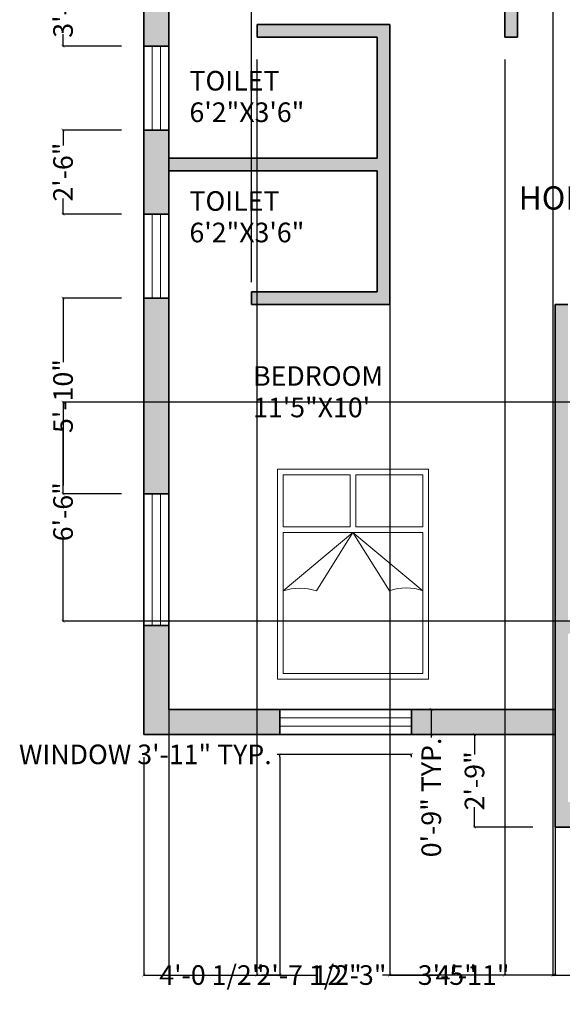
# Model space of a CAD drawing. Units: inches. Extents: x 98 to 545, y 56 to 703.
# Tile 1 of 4: x 98 to 292, y 56 to 408. Entities that reach past the tile are written whole.
import ezdxf

# ---------------------------------------------------------------- set-up
doc = ezdxf.new("R2010")
doc.units = ezdxf.units.IN
doc.header["$MEASUREMENT"] = 0
for name, color, linetype, lineweight in [('A-ANNO-DIMS', 2, 'Continuous', 18), ('A-ANNO-TEXT', 7, 'Continuous', 25), ('A-AREA-IDEN', 7, 'Continuous', 25), ('A-GLAZ', 4, 'Continuous', 18), ('A-WALL', 7, 'Continuous', 35), ('Furniture', 7, 'Continuous', 15)]:
    doc.layers.add(name, color=color, linetype=linetype, lineweight=lineweight)
doc.layers.add('A-WALL-PATT', color=18, linetype='Continuous', lineweight=13, true_color=0x000000)
doc.styles.get("Standard").update_dxf_attribs({"font": 'arial.ttf'})
doc.dimstyles.get("Standard").update_dxf_attribs({"dimtxt": 7, "dimasz": 1, "dimexe": 0.183, "dimexo": 8, "dimgap": 0.09, "dimtad": 0, "dimdec": 4, "dimzin": 0, "dimdsep": 46, "dimlunit": 3, "dimtxsty": 'Standard', "dimblk": 'ARCHTICK', "dimcen": 0, "dimclrd": 253, "dimclre": 251, "dimadec": 0, "dimazin": 0, "dimtfac": 1, "dimtdec": 4, "dimtofl": 0, "dimtmove": 0, "dimatfit": 3, "dimfxl": 1, "dimtolj": 1, "dimtzin": 0, "dimarcsym": 0})

# ---------------------------------------------------------------- blocks, each defined once
blk = doc.blocks.new('WIN-SASH-47IN')
for p, q in [((47, 9), (0, 9)), ((0, 6), (47, 6)), ((0, 3), (47, 3)), ((0, 0), (47, 0))]:
    blk.add_line(p, q)
blk = doc.blocks.new('WIN-SASH-30IN')
for p, q in [((30, 9), (0, 9)), ((0, 6), (30, 6)), ((0, 3), (30, 3)), ((0, 0), (30, 0))]:
    blk.add_line(p, q)
blk = doc.blocks.new('_ArchTick')
at = {"color": 0, "linetype": 'ByBlock', "const_width": 0.15}
blk.add_lwpolyline([(-0.5, -0.5), (0.5, 0.5)], dxfattribs=at)
blk = doc.blocks.new('*D9')
at = {"layer": 'A-ANNO-DIMS', "color": 253, "lineweight": -2, "transparency": 16777216}
for p, q in [((191.02, 145.65), (190.02, 145.65)), ((238.02, 145.65), (191.02, 145.65))]:
    blk.add_line(p, q, dxfattribs=at)
at = {"layer": 'A-ANNO-DIMS', "color": 251, "lineweight": -2, "transparency": 16777216}
for p, q in [((191.02, 144.7), (191.02, 145.46)), ((238.02, 144.7), (238.02, 145.46))]:
    blk.add_line(p, q, dxfattribs=at)
at = {"layer": 'Defpoints', "color": 0, "transparency": 16777216}
for p in [(191.02, 152.7), (238.02, 152.7), (191.02, 145.65)]:
    blk.add_point(p, dxfattribs=at)
at = {"layer": 'A-ANNO-DIMS', "color": 253, "lineweight": -2, "transparency": 16777216, "rotation": 180}
blk.add_blockref('_ArchTick', (191.02, 145.65), dxfattribs=at)
at = {"layer": 'A-ANNO-DIMS', "color": 253, "lineweight": -2, "transparency": 16777216}
blk.add_blockref('_ArchTick', (238.02, 145.65), dxfattribs=at)
at = {"layer": 'A-ANNO-DIMS', "color": 0, "transparency": 16777216, "insert": (142.92, 145.65), "char_height": 7, "attachment_point": 5}
blk.add_mtext('\\A1;WINDOW 3\'-11" TYP.', dxfattribs=at)
blk = doc.blocks.new('*D10')
at = {"layer": 'A-ANNO-DIMS', "color": 253, "lineweight": -2, "transparency": 16777216}
for p, q in [((245.07, 161.7), (245.07, 152.7)), ((245.07, 152.7), (245.07, 151.7))]:
    blk.add_line(p, q, dxfattribs=at)
at = {"layer": 'A-ANNO-DIMS', "color": 251, "lineweight": -2, "transparency": 16777216}
for p, q in [((246.02, 161.7), (245.25, 161.7)), ((246.02, 152.7), (245.25, 152.7))]:
    blk.add_line(p, q, dxfattribs=at)
at = {"layer": 'Defpoints', "color": 0, "transparency": 16777216}
for p in [(238.02, 161.7), (238.02, 152.7), (245.07, 152.7)]:
    blk.add_point(p, dxfattribs=at)
at = {"layer": 'A-ANNO-DIMS', "color": 253, "lineweight": -2, "transparency": 16777216}
for p, rotation in [((245.07, 161.7), 90), ((245.07, 152.7), 270)]:
    blk.add_blockref('_ArchTick', p, dxfattribs=dict(at, rotation=rotation))
at = {"layer": 'A-ANNO-DIMS', "color": 0, "transparency": 16777216, "insert": (245.07, 130.27), "char_height": 7, "attachment_point": 5, "rotation": 90}
blk.add_mtext('\\A1;0\'-9" TYP.', dxfattribs=at)
blk = doc.blocks.new('*D18')
at = {"layer": 'A-ANNO-DIMS', "color": 251, "lineweight": -2, "transparency": 16777216}
for p, q in [((142.36, 144.7), (142.36, 66.66)), ((191.02, 144.7), (191.02, 66.66))]:
    blk.add_line(p, q, dxfattribs=at)
at = {"layer": 'A-ANNO-DIMS', "color": 253, "lineweight": -2, "transparency": 16777216}
for p, q in [((142.36, 66.85), (149, 66.85)), ((191.02, 66.85), (184.38, 66.85))]:
    blk.add_line(p, q, dxfattribs=at)
at = {"layer": 'Defpoints', "color": 0, "transparency": 16777216}
for p in [(142.36, 152.7), (191.02, 152.7), (191.02, 66.85)]:
    blk.add_point(p, dxfattribs=at)
at = {"layer": 'A-ANNO-DIMS', "color": 253, "lineweight": -2, "transparency": 16777216, "rotation": 180}
blk.add_blockref('_ArchTick', (142.36, 66.85), dxfattribs=at)
at = {"layer": 'A-ANNO-DIMS', "color": 253, "lineweight": -2, "transparency": 16777216}
blk.add_blockref('_ArchTick', (191.02, 66.85), dxfattribs=at)
at = {"layer": 'A-ANNO-DIMS', "color": 0, "transparency": 16777216, "insert": (166.69, 66.85), "char_height": 7, "attachment_point": 5}
blk.add_mtext('\\A1;4\'-0 1/2"', dxfattribs=at)
blk = doc.blocks.new('*D19')
at = {"layer": 'A-ANNO-DIMS', "color": 251, "lineweight": -2, "transparency": 16777216}
for p, q in [((142.36, 144.7), (142.36, 66.66)), ((289.36, 144.7), (289.36, 66.66))]:
    blk.add_line(p, q, dxfattribs=at)
at = {"layer": 'A-ANNO-DIMS', "color": 253, "lineweight": -2, "transparency": 16777216}
for p, q in [((142.36, 66.85), (204.08, 66.85)), ((289.36, 66.85), (227.65, 66.85))]:
    blk.add_line(p, q, dxfattribs=at)
at = {"layer": 'Defpoints', "color": 0, "transparency": 16777216}
for p in [(142.36, 152.7), (289.36, 152.7), (289.36, 66.85)]:
    blk.add_point(p, dxfattribs=at)
at = {"layer": 'A-ANNO-DIMS', "color": 253, "lineweight": -2, "transparency": 16777216, "rotation": 180}
blk.add_blockref('_ArchTick', (142.36, 66.85), dxfattribs=at)
at = {"layer": 'A-ANNO-DIMS', "color": 253, "lineweight": -2, "transparency": 16777216}
blk.add_blockref('_ArchTick', (289.36, 66.85), dxfattribs=at)
at = {"layer": 'A-ANNO-DIMS', "color": 0, "transparency": 16777216, "insert": (215.86, 66.85), "char_height": 7, "attachment_point": 5}
blk.add_mtext('\\A1;12\'-3"', dxfattribs=at)
blk = doc.blocks.new('*D20')
at = {"layer": 'A-ANNO-DIMS', "color": 251, "lineweight": -2, "transparency": 16777216}
for p, q in [((281.36, 152.7), (260.33, 152.7)), ((281.36, 119.7), (260.33, 119.7))]:
    blk.add_line(p, q, dxfattribs=at)
at = {"layer": 'A-ANNO-DIMS', "color": 253, "lineweight": -2, "transparency": 16777216}
for p, q in [((260.51, 152.7), (260.51, 145.65)), ((260.51, 119.7), (260.51, 126.74))]:
    blk.add_line(p, q, dxfattribs=at)
at = {"layer": 'Defpoints', "color": 0, "transparency": 16777216}
for p in [(260.51, 152.7), (289.36, 152.7), (289.36, 119.7)]:
    blk.add_point(p, dxfattribs=at)
at = {"layer": 'A-ANNO-DIMS', "color": 253, "lineweight": -2, "transparency": 16777216}
for p, rotation in [((260.51, 152.7), 90), ((260.51, 119.7), 270)]:
    blk.add_blockref('_ArchTick', p, dxfattribs=dict(at, rotation=rotation))
at = {"layer": 'A-ANNO-DIMS', "color": 0, "transparency": 16777216, "insert": (260.51, 136.2), "char_height": 7, "attachment_point": 5, "rotation": 90}
blk.add_mtext('\\A1;2\'-9"', dxfattribs=at)
blk = doc.blocks.new('*D27')
at = {"layer": 'A-ANNO-DIMS', "color": 251, "lineweight": -2, "transparency": 16777216}
for p, q in [((134.36, 442.08), (113.33, 442.08)), ((134.36, 398.55), (113.33, 398.55))]:
    blk.add_line(p, q, dxfattribs=at)
at = {"layer": 'A-ANNO-DIMS', "color": 253, "lineweight": -2, "transparency": 16777216}
for p, q in [((113.51, 442.08), (113.51, 437.86)), ((113.51, 398.55), (113.51, 402.77))]:
    blk.add_line(p, q, dxfattribs=at)
at = {"layer": 'Defpoints', "color": 0, "transparency": 16777216}
for p in [(142.36, 442.08), (113.51, 398.55), (142.36, 398.55)]:
    blk.add_point(p, dxfattribs=at)
at = {"layer": 'A-ANNO-DIMS', "color": 253, "lineweight": -2, "transparency": 16777216}
for p, rotation in [((113.51, 442.08), 90), ((113.51, 398.55), 270)]:
    blk.add_blockref('_ArchTick', p, dxfattribs=dict(at, rotation=rotation))
at = {"layer": 'A-ANNO-DIMS', "color": 0, "transparency": 16777216, "insert": (113.51, 420.32), "char_height": 7, "attachment_point": 5, "rotation": 90}
blk.add_mtext('\\A1;3\'-7 1/2"', dxfattribs=at)
blk = doc.blocks.new('*D28')
at = {"layer": 'A-ANNO-DIMS', "color": 251, "lineweight": -2, "transparency": 16777216}
for p, q in [((134.36, 368.55), (113.33, 368.55)), ((134.36, 338.55), (113.33, 338.55))]:
    blk.add_line(p, q, dxfattribs=at)
at = {"layer": 'A-ANNO-DIMS', "color": 253, "lineweight": -2, "transparency": 16777216}
for p, q in [((113.51, 368.55), (113.51, 363)), ((113.51, 338.55), (113.51, 344.1))]:
    blk.add_line(p, q, dxfattribs=at)
at = {"layer": 'Defpoints', "color": 0, "transparency": 16777216}
for p in [(142.36, 368.55), (113.51, 338.55), (142.36, 338.55)]:
    blk.add_point(p, dxfattribs=at)
at = {"layer": 'A-ANNO-DIMS', "color": 253, "lineweight": -2, "transparency": 16777216}
for p, rotation in [((113.51, 368.55), 90), ((113.51, 338.55), 270)]:
    blk.add_blockref('_ArchTick', p, dxfattribs=dict(at, rotation=rotation))
at = {"layer": 'A-ANNO-DIMS', "color": 0, "transparency": 16777216, "insert": (113.51, 353.55), "char_height": 7, "attachment_point": 5, "rotation": 90}
blk.add_mtext('\\A1;2\'-6"', dxfattribs=at)
blk = doc.blocks.new('*D29')
at = {"layer": 'A-ANNO-DIMS', "color": 251, "lineweight": -2, "transparency": 16777216}
for p, q in [((134.36, 308.55), (113.33, 308.55)), ((134.36, 238.66), (113.33, 238.66))]:
    blk.add_line(p, q, dxfattribs=at)
at = {"layer": 'A-ANNO-DIMS', "color": 253, "lineweight": -2, "transparency": 16777216}
for p, q in [((113.51, 308.55), (113.51, 285.72)), ((113.51, 238.66), (113.51, 261.49))]:
    blk.add_line(p, q, dxfattribs=at)
at = {"layer": 'Defpoints', "color": 0, "transparency": 16777216}
for p in [(142.36, 308.55), (113.51, 238.66), (142.36, 238.66)]:
    blk.add_point(p, dxfattribs=at)
at = {"layer": 'A-ANNO-DIMS', "color": 253, "lineweight": -2, "transparency": 16777216}
for p, rotation in [((113.51, 308.55), 90), ((113.51, 238.66), 270)]:
    blk.add_blockref('_ArchTick', p, dxfattribs=dict(at, rotation=rotation))
at = {"layer": 'A-ANNO-DIMS', "color": 0, "transparency": 16777216, "insert": (113.51, 273.6), "char_height": 7, "attachment_point": 5, "rotation": 90}
blk.add_mtext('\\A1;5\'-10"', dxfattribs=at)
blk = doc.blocks.new('*D33')
at = {"layer": 'A-ANNO-DIMS', "color": 251, "lineweight": -2, "transparency": 16777216}
for p, q in [((485.36, 271.39), (113.33, 271.39)), ((485.36, 193.2), (113.33, 193.2))]:
    blk.add_line(p, q, dxfattribs=at)
at = {"layer": 'A-ANNO-DIMS', "color": 253, "lineweight": -2, "transparency": 16777216}
for p, q in [((113.51, 271.39), (113.51, 241.7)), ((113.51, 193.2), (113.51, 222.88))]:
    blk.add_line(p, q, dxfattribs=at)
at = {"layer": 'Defpoints', "color": 0, "transparency": 16777216}
for p in [(493.36, 271.39), (113.51, 193.2), (493.36, 193.2)]:
    blk.add_point(p, dxfattribs=at)
at = {"layer": 'A-ANNO-DIMS', "color": 253, "lineweight": -2, "transparency": 16777216}
for p, rotation in [((113.51, 271.39), 90), ((113.51, 193.2), 270)]:
    blk.add_blockref('_ArchTick', p, dxfattribs=dict(at, rotation=rotation))
at = {"layer": 'A-ANNO-DIMS', "color": 0, "transparency": 16777216, "insert": (113.51, 232.29), "char_height": 7, "attachment_point": 5, "rotation": 90}
blk.add_mtext('\\A1;6\'-6"', dxfattribs=at)
blk = doc.blocks.new('*D40')
at = {"layer": 'A-ANNO-DIMS', "color": 251, "lineweight": -2, "transparency": 16777216}
for p, q in [((151.36, 393.7), (151.36, 66.66)), ((182.81, 393.7), (182.81, 66.66))]:
    blk.add_line(p, q, dxfattribs=at)
at = {"layer": 'A-ANNO-DIMS', "color": 253, "lineweight": -2, "transparency": 16777216}
for p, q in [((151.36, 66.85), (182.81, 66.85)), ((182.81, 66.85), (183.81, 66.85))]:
    blk.add_line(p, q, dxfattribs=at)
at = {"layer": 'Defpoints', "color": 0, "transparency": 16777216}
for p in [(151.36, 401.7), (182.81, 401.7), (182.81, 66.85)]:
    blk.add_point(p, dxfattribs=at)
at = {"layer": 'A-ANNO-DIMS', "color": 253, "lineweight": -2, "transparency": 16777216, "rotation": 180}
blk.add_blockref('_ArchTick', (151.36, 66.85), dxfattribs=at)
at = {"layer": 'A-ANNO-DIMS', "color": 253, "lineweight": -2, "transparency": 16777216}
blk.add_blockref('_ArchTick', (182.81, 66.85), dxfattribs=at)
at = {"layer": 'A-ANNO-DIMS', "color": 0, "transparency": 16777216, "insert": (201.42, 66.85), "char_height": 7, "attachment_point": 5}
blk.add_mtext('\\A1;2\'-7 1/2"', dxfattribs=at)
blk = doc.blocks.new('*D41')
at = {"layer": 'A-ANNO-DIMS', "color": 251, "lineweight": -2, "transparency": 16777216}
for p, q in [((151.36, 314.3), (151.36, 688.73)), ((180.85, 314.3), (180.85, 688.73))]:
    blk.add_line(p, q, dxfattribs=at)
at = {"layer": 'A-ANNO-DIMS', "color": 253, "lineweight": -2, "transparency": 16777216}
for p, q in [((151.36, 688.55), (180.85, 688.55)), ((180.85, 688.55), (181.85, 688.55))]:
    blk.add_line(p, q, dxfattribs=at)
at = {"layer": 'Defpoints', "color": 0, "transparency": 16777216}
for p in [(180.85, 688.55), (151.36, 306.3), (180.85, 306.3)]:
    blk.add_point(p, dxfattribs=at)
at = {"layer": 'A-ANNO-DIMS', "color": 253, "lineweight": -2, "transparency": 16777216, "rotation": 180}
blk.add_blockref('_ArchTick', (151.36, 688.55), dxfattribs=at)
at = {"layer": 'A-ANNO-DIMS', "color": 253, "lineweight": -2, "transparency": 16777216}
blk.add_blockref('_ArchTick', (180.85, 688.55), dxfattribs=at)
at = {"layer": 'A-ANNO-DIMS', "color": 0, "transparency": 16777216, "insert": (199.46, 688.55), "char_height": 7, "attachment_point": 5}
blk.add_mtext('\\A1;2\'-5 1/2"', dxfattribs=at)
blk = doc.blocks.new('*D42')
at = {"layer": 'A-ANNO-DIMS', "color": 251, "lineweight": -2, "transparency": 16777216}
for p, q in [((288.56, 558.2), (288.56, 66.66)), ((321.46, 558.2), (321.46, 66.66))]:
    blk.add_line(p, q, dxfattribs=at)
at = {"layer": 'A-ANNO-DIMS', "color": 253, "lineweight": -2, "transparency": 16777216}
for p, q in [((288.56, 66.85), (295.56, 66.85)), ((321.46, 66.85), (314.46, 66.85))]:
    blk.add_line(p, q, dxfattribs=at)
at = {"layer": 'Defpoints', "color": 0, "transparency": 16777216}
for p in [(288.56, 566.2), (321.46, 566.2), (321.46, 66.85)]:
    blk.add_point(p, dxfattribs=at)
at = {"layer": 'A-ANNO-DIMS', "color": 253, "lineweight": -2, "transparency": 16777216, "rotation": 180}
blk.add_blockref('_ArchTick', (288.56, 66.85), dxfattribs=at)
at = {"layer": 'A-ANNO-DIMS', "color": 253, "lineweight": -2, "transparency": 16777216}
blk.add_blockref('_ArchTick', (321.46, 66.85), dxfattribs=at)
at = {"layer": 'A-ANNO-DIMS', "color": 0, "transparency": 16777216, "insert": (305.01, 66.85), "char_height": 7, "attachment_point": 5}
blk.add_mtext('\\A1;2\'-9"', dxfattribs=at)
blk = doc.blocks.new('*D45')
at = {"layer": 'A-ANNO-DIMS', "color": 251, "lineweight": -2, "transparency": 16777216}
for p, q in [((230.26, 398.2), (230.26, 66.66)), ((271.36, 393.7), (271.36, 66.66))]:
    blk.add_line(p, q, dxfattribs=at)
at = {"layer": 'A-ANNO-DIMS', "color": 253, "lineweight": -2, "transparency": 16777216}
for p, q in [((230.26, 66.85), (241.42, 66.85)), ((271.36, 66.85), (260.21, 66.85))]:
    blk.add_line(p, q, dxfattribs=at)
at = {"layer": 'Defpoints', "color": 0, "transparency": 16777216}
for p in [(230.26, 406.2), (271.36, 401.7), (271.36, 66.85)]:
    blk.add_point(p, dxfattribs=at)
at = {"layer": 'A-ANNO-DIMS', "color": 253, "lineweight": -2, "transparency": 16777216, "rotation": 180}
blk.add_blockref('_ArchTick', (230.26, 66.85), dxfattribs=at)
at = {"layer": 'A-ANNO-DIMS', "color": 253, "lineweight": -2, "transparency": 16777216}
blk.add_blockref('_ArchTick', (271.36, 66.85), dxfattribs=at)
at = {"layer": 'A-ANNO-DIMS', "color": 0, "transparency": 16777216, "insert": (250.81, 66.85), "char_height": 7, "attachment_point": 5}
blk.add_mtext('\\A1;3\'-5"', dxfattribs=at)
blk = doc.blocks.new('*D46')
at = {"layer": 'A-ANNO-DIMS', "color": 251, "lineweight": -2, "transparency": 16777216}
for p, q in [((230.26, 298.3), (230.26, 66.66)), ((289.36, 298.3), (289.36, 66.66))]:
    blk.add_line(p, q, dxfattribs=at)
at = {"layer": 'A-ANNO-DIMS', "color": 253, "lineweight": -2, "transparency": 16777216}
for p, q in [((230.26, 66.85), (247.56, 66.85)), ((289.36, 66.85), (272.07, 66.85))]:
    blk.add_line(p, q, dxfattribs=at)
at = {"layer": 'Defpoints', "color": 0, "transparency": 16777216}
for p in [(230.26, 306.3), (289.36, 306.3), (289.36, 66.85)]:
    blk.add_point(p, dxfattribs=at)
at = {"layer": 'A-ANNO-DIMS', "color": 253, "lineweight": -2, "transparency": 16777216, "rotation": 180}
blk.add_blockref('_ArchTick', (230.26, 66.85), dxfattribs=at)
at = {"layer": 'A-ANNO-DIMS', "color": 253, "lineweight": -2, "transparency": 16777216}
blk.add_blockref('_ArchTick', (289.36, 66.85), dxfattribs=at)
at = {"layer": 'A-ANNO-DIMS', "color": 0, "transparency": 16777216, "insert": (259.81, 66.85), "char_height": 7, "attachment_point": 5}
blk.add_mtext('\\A1;4\'-11"', dxfattribs=at)
blk = doc.blocks.new('*D47')
at = {"layer": 'A-ANNO-DIMS', "color": 251, "lineweight": -2, "transparency": 16777216}
for p, q in [((271.36, 409.7), (271.36, 688.73)), ((275.86, 409.7), (275.86, 688.73))]:
    blk.add_line(p, q, dxfattribs=at)
at = {"layer": 'A-ANNO-DIMS', "color": 253, "lineweight": -2, "transparency": 16777216}
for p, q in [((271.36, 688.55), (275.86, 688.55)), ((275.86, 688.55), (276.86, 688.55))]:
    blk.add_line(p, q, dxfattribs=at)
at = {"layer": 'Defpoints', "color": 0, "transparency": 16777216}
for p in [(275.86, 688.55), (271.36, 401.7), (275.86, 401.7)]:
    blk.add_point(p, dxfattribs=at)
at = {"layer": 'A-ANNO-DIMS', "color": 253, "lineweight": -2, "transparency": 16777216, "rotation": 180}
blk.add_blockref('_ArchTick', (271.36, 688.55), dxfattribs=at)
at = {"layer": 'A-ANNO-DIMS', "color": 253, "lineweight": -2, "transparency": 16777216}
blk.add_blockref('_ArchTick', (275.86, 688.55), dxfattribs=at)
at = {"layer": 'A-ANNO-DIMS', "color": 0, "transparency": 16777216, "insert": (294.41, 688.55), "char_height": 7, "attachment_point": 5}
blk.add_mtext('\\A1;0\'-4 1/2"', dxfattribs=at)

msp = doc.modelspace()

# ---------------------------------------------------------------- hatches: boundary and pattern name
at = {"layer": 'A-WALL-PATT'}
h = msp.add_hatch(color=256, dxfattribs=at)
h.dxf.hatch_style = 1
h.paths.add_polyline_path([(173.39577, 659.69681), (142.36469, 659.69681), (142.36469, 612.44216), (151.36469, 612.44216), (151.36469, 650.69681), (173.39577, 650.69681)])
h.paths.add_polyline_path([(282.86266, 659.69681), (220.39577, 659.69681), (220.39577, 650.69681), (271.36469, 650.69681), (271.36469, 566.19681), (275.86469, 566.19681), (288.55623, 566.19681), (288.55623, 570.69681), (275.86469, 570.69681), (275.86469, 650.69681), (282.86266, 650.69681)])
h.paths.add_polyline_path([(358.82163, 659.69681), (312.86266, 659.69681), (312.86266, 650.69681), (321.46469, 650.69681), (321.46469, 570.69681), (321.46469, 566.19681), (321.46469, 530.69681), (321.46469, 526.19681), (325.96469, 526.19681), (325.96469, 530.69681), (325.96469, 650.69681), (358.82163, 650.69681)])
h.paths.add_polyline_path([(451.98971, 659.69681), (405.82163, 659.69681), (405.82163, 650.69681), (435.16469, 650.69681), (435.16469, 570.08746), (439.66469, 570.08746), (439.66469, 650.69681), (451.98971, 650.69681)])
h.paths.add_polyline_path([(502.36469, 659.69681), (481.98971, 659.69681), (481.98971, 650.69681), (493.36469, 650.69681), (493.36469, 614.57752), (502.36469, 614.57752)])
h.paths.add_polyline_path([(502.36469, 579.57752), (493.36469, 579.57752), (493.36469, 530.69681), (439.66469, 530.69681), (435.16469, 530.69681), (373.81242, 530.69681), (373.81242, 526.19681), (493.36469, 526.19681), (493.36469, 480.62471), (502.36469, 480.62471)])
h.paths.add_polyline_path([(502.36469, 445.62471), (493.36469, 445.62471), (493.36469, 406.19681), (493.36469, 401.69681), (493.36469, 397.69681), (379.47742, 397.69681), (379.47742, 393.19681), (493.36469, 393.19681), (493.36469, 306.38501), (502.36469, 306.38501)])
h.paths.add_polyline_path([(502.36469, 271.385), (493.36469, 271.385), (493.36469, 193.19681), (478.76571, 193.19681), (478.76571, 188.69681), (493.36469, 188.69681), (493.36469, 128.69681), (487.75103, 128.69681), (487.75103, 119.69681), (502.36469, 119.69681)])
h.paths.add_polyline_path([(452.75103, 128.69681), (445.36469, 128.69681), (445.36469, 188.69681), (456.12508, 188.69681), (456.12508, 193.19681), (440.86469, 193.19681), (440.86469, 119.69681), (452.75103, 119.69681)])
h.paths.add_polyline_path([(307.21941, 128.69681), (293.86469, 128.69681), (293.86469, 188.69681), (404.74827, 188.69681), (404.74827, 193.19681), (293.86469, 193.19681), (293.86469, 306.29681), (289.36469, 306.29681), (289.36469, 119.69681), (307.21941, 119.69681)])
h.paths.add_polyline_path([(289.36469, 161.69681), (238.02122, 161.69681), (238.02122, 152.69681), (289.36469, 152.69681)])
h.paths.add_polyline_path([(191.02122, 161.69681), (151.36469, 161.69681), (151.36469, 191.65928), (142.36469, 191.65928), (142.36469, 152.69681), (151.36469, 152.69681), (191.02122, 152.69681)])
h.paths.add_polyline_path([(151.36469, 306.29681), (151.36469, 308.54862), (142.36469, 308.54862), (142.36469, 238.65928), (151.36469, 238.65928)])
h.paths.add_polyline_path([(230.26469, 401.69681), (230.26469, 406.19681), (182.81458, 406.19681), (182.81458, 401.69681), (225.76469, 401.69681), (225.76469, 358.49681), (151.36469, 358.49681), (151.36469, 368.55378), (142.36469, 368.55378), (142.36469, 338.54862), (151.36469, 338.54862), (151.36469, 353.99681), (225.76469, 353.99681), (225.76469, 310.79681), (180.84919, 310.79681), (180.84919, 306.29681), (230.26469, 306.29681)])
h.paths.add_polyline_path([(151.36469, 442.07867), (142.36469, 442.07867), (142.36469, 398.55378), (151.36469, 398.55378), (151.36469, 401.69681)])
h.paths.add_polyline_path([(151.36469, 526.19681), (271.36469, 526.19681), (271.36469, 406.19681), (271.36469, 401.69681), (275.86469, 401.69681), (275.86469, 406.19681), (275.86469, 526.19681), (275.86469, 530.69681), (271.36469, 530.69681), (151.36469, 530.69681), (151.36469, 565.44216), (142.36469, 565.44216), (142.36469, 489.07867), (151.36469, 489.07867)])

# ---------------------------------------------------------------- linework, layer by layer
at = {"layer": 'A-WALL'}
for p, q in [((142.36469, 659.69681), (142.36469, 152.69681)), ((151.36469, 526.19681), (151.36469, 401.69681)), ((271.36469, 526.19681), (271.36469, 406.19681)), ((275.86469, 526.19681), (275.86469, 406.19681)), ((230.26469, 406.19681), (182.81458, 406.19681)), ((182.81458, 406.19681), (182.81458, 401.69681)), ((230.26469, 401.69681), (230.26469, 406.19681)), ((271.36469, 406.19681), (271.36469, 401.69681)), ((275.86469, 406.19681), (275.86469, 401.69681)), ((151.36469, 401.69681), (151.36469, 358.49681)), ((225.76469, 401.69681), (182.81458, 401.69681)), ((225.76469, 401.69681), (225.76469, 358.49681)), ((230.26469, 401.69681), (230.26469, 306.29681)), ((275.86469, 401.69681), (271.36469, 401.69681)), ((142.36469, 398.55378), (151.36469, 398.55378)), ((151.36469, 368.55378), (142.36469, 368.55378)), ((225.76469, 358.49681), (151.36469, 358.49681)), ((225.76469, 353.99681), (151.36469, 353.99681)), ((151.36469, 353.99681), (151.36469, 310.79681)), ((225.76469, 353.99681), (225.76469, 310.79681)), ((142.36469, 338.54862), (151.36469, 338.54862)), ((151.36469, 306.29681), (151.36469, 310.79681)), ((225.76469, 310.79681), (180.84919, 310.79681)), ((180.84919, 310.79681), (180.84919, 306.29681)), ((151.36469, 308.54862), (142.36469, 308.54862)), ((151.36469, 306.29681), (151.36469, 161.69681)), ((230.26469, 306.29681), (180.84919, 306.29681)), ((289.36469, 306.29681), (289.36469, 119.69681)), ((293.86469, 306.29681), (289.36469, 306.29681)), ((142.36469, 238.65928), (151.36469, 238.65928)), ((151.36469, 191.65928), (142.36469, 191.65928)), ((151.36469, 161.69681), (289.36469, 161.69681)), ((191.02122, 161.69681), (191.02122, 152.69681)), ((238.02122, 152.69681), (238.02122, 161.69681)), ((151.36469, 152.69681), (142.36469, 152.69681)), ((151.36469, 152.69681), (289.36469, 152.69681)), ((289.36469, 119.69681), (502.36469, 119.69681))]:
    msp.add_line(p, q, dxfattribs=at)
at = {"layer": 'Furniture'}
for p, q in [((190.10428, 247.48939), (244.10428, 247.48939)), ((190.10428, 172.48939), (190.10428, 247.48939)), ((244.10428, 247.48939), (244.10428, 172.48939)), ((192.10428, 245.48939), (216.10428, 245.48939)), ((192.10428, 226.91399), (192.10428, 245.48939)), ((216.10428, 226.91399), (216.10428, 245.48939)), ((218.10428, 226.91399), (218.10428, 245.48939)), ((218.10428, 245.48939), (242.10428, 245.48939)), ((242.10428, 245.48939), (242.10428, 226.91399)), ((192.10428, 226.91399), (216.10428, 226.91399)), ((218.10428, 226.91399), (242.10428, 226.91399)), ((192.10428, 174.48939), (192.10428, 224.91399)), ((192.10428, 224.91399), (242.10428, 224.91399)), ((217.10428, 224.91399), (192.10428, 204.00203)), ((204.10428, 204.00203), (217.10428, 224.91399)), ((217.10428, 224.91399), (242.10428, 204.00203)), ((230.10428, 204.00203), (217.10428, 224.91399)), ((242.10428, 224.91399), (242.10428, 174.48939)), ((244.10428, 172.48939), (190.10428, 172.48939)), ((242.10428, 174.48939), (192.10428, 174.48939))]:
    msp.add_line(p, q, dxfattribs=at)
for centre, radius, start, end in [((198.10428, 185.53949), 19.41302, 71.9967481, 108.0032519), ((236.10428, 188.25457), 16.85178, 69.1424643, 110.8575357)]:
    msp.add_arc(centre, radius, start, end, dxfattribs=at)

# ---------------------------------------------------------------- block references
at = {"layer": 'A-GLAZ'}
for name, p, rotation in [('WIN-SASH-30IN', (151.3645, 368.55411), 89.99999999999999), ('WIN-SASH-30IN', (151.3645, 308.54896), 89.99999999999991), ('WIN-SASH-47IN', (151.3645, 191.65965), 89.99999999999967), ('WIN-SASH-47IN', (238.02085, 161.69661), 180)]:
    msp.add_blockref(name, p, dxfattribs=dict(at, rotation=rotation))

# ---------------------------------------------------------------- texts
at = {"layer": 'A-ANNO-TEXT'}
msp.add_text('HOME', height=8.320668, dxfattribs=at).set_placement((276.29482, 340.16056))
at = {"layer": 'A-AREA-IDEN'}
for s, p in [('TOILET', (158.68817, 382.6768)), ('6\'2"X3\'6"', (158.68817, 371.43192)), ('TOILET', (158.68817, 339.7276)), ('6\'2"X3\'6"', (158.68817, 328.48271)), ('BEDROOM', (181.41646, 277.2582)), ('11\'5"X10\'', (181.41646, 266.01331))]:
    msp.add_text(s, height=7, dxfattribs=at).set_placement(p)

# ---------------------------------------------------------------- dimensions: what is measured, and where the dimension line sits
at = {"layer": 'A-ANNO-DIMS'}
for base, p1, p2, picture, middle in [((180.84919, 688.54681), (151.36469, 306.29681), (180.84919, 306.29681), '*D41', (199.45829, 688.54681)), ((275.86469, 688.54681), (271.36469, 401.69681), (275.86469, 401.69681), '*D47', (294.41411, 688.54681)), ((321.46469, 66.84681), (288.55623, 566.19681), (321.46469, 566.19681), '*D42', (305.01046, 66.84681)), ((271.36469, 66.84681), (230.26469, 406.19681), (271.36469, 401.69681), '*D45', (250.81469, 66.84681)), ((182.81458, 66.84681), (151.36469, 401.69681), (182.81458, 401.69681), '*D40', (201.42368, 66.84681)), ((289.36469, 66.84681), (230.26469, 306.29681), (289.36469, 306.29681), '*D46', (259.81469, 66.84681)), ((191.02122, 66.84681), (142.36469, 152.69681), (191.02122, 152.69681), '*D18', (166.69296, 66.84681)), ((289.36469, 66.84681), (142.36469, 152.69681), (289.36469, 152.69681), '*D19', (215.86469, 66.84681))]:
    dim = msp.add_linear_dim(base=base, p1=p1, p2=p2, dimstyle='Standard', override={"dimdec": 1, "dimlfac": 1, "dimrnd": 0, "dimzin": 1, "dimdsep": 46, "dimlunit": 4, "dimfrac": 2}, dxfattribs=at)
    dim.commit()
    dim.dimension.update_dxf_attribs({"geometry": picture, "text_midpoint": middle})
for base, p1, p2, picture, middle in [((113.51469, 398.55378), (142.36469, 442.07867), (142.36469, 398.55378), '*D27', (113.51469, 420.31622)), ((113.51469, 338.54862), (142.36469, 368.55378), (142.36469, 338.54862), '*D28', (113.51469, 353.5512)), ((113.51469, 238.65928), (142.36469, 308.54862), (142.36469, 238.65928), '*D29', (113.51469, 273.60395)), ((113.51469, 193.19681), (493.36469, 271.385), (493.36469, 193.19681), '*D33', (113.51469, 232.29091)), ((260.51469, 152.69681), (289.36469, 119.69681), (289.36469, 152.69681), '*D20', (260.51469, 136.19681))]:
    dim = msp.add_linear_dim(base=base, p1=p1, p2=p2, angle=90, dimstyle='Standard', override={"dimdec": 1, "dimlfac": 1, "dimrnd": 0, "dimzin": 1, "dimdsep": 46, "dimlunit": 4, "dimfrac": 2}, dxfattribs=at)
    dim.commit()
    dim.dimension.update_dxf_attribs({"geometry": picture, "text_midpoint": middle})
for base, p1, p2, angle, text, picture, middle in [((191.02122, 145.64681), (238.02122, 152.69681), (191.02122, 152.69681), 180, 'WINDOW <> TYP.', '*D9', (142.92235, 145.64681)), ((245.07122, 152.69681), (238.02122, 161.69681), (238.02122, 152.69681), 270, '<> TYP.', '*D10', (245.07122, 130.27256))]:
    dim = msp.add_linear_dim(base=base, p1=p1, p2=p2, angle=angle, text=text, dimstyle='Standard', override={"dimdec": 1, "dimlfac": 1, "dimrnd": 0, "dimzin": 1, "dimdsep": 46, "dimlunit": 4, "dimfrac": 2}, dxfattribs=at)
    dim.commit()
    dim.dimension.update_dxf_attribs({"geometry": picture, "text_midpoint": middle})

doc.saveas('drawing.dxf')
